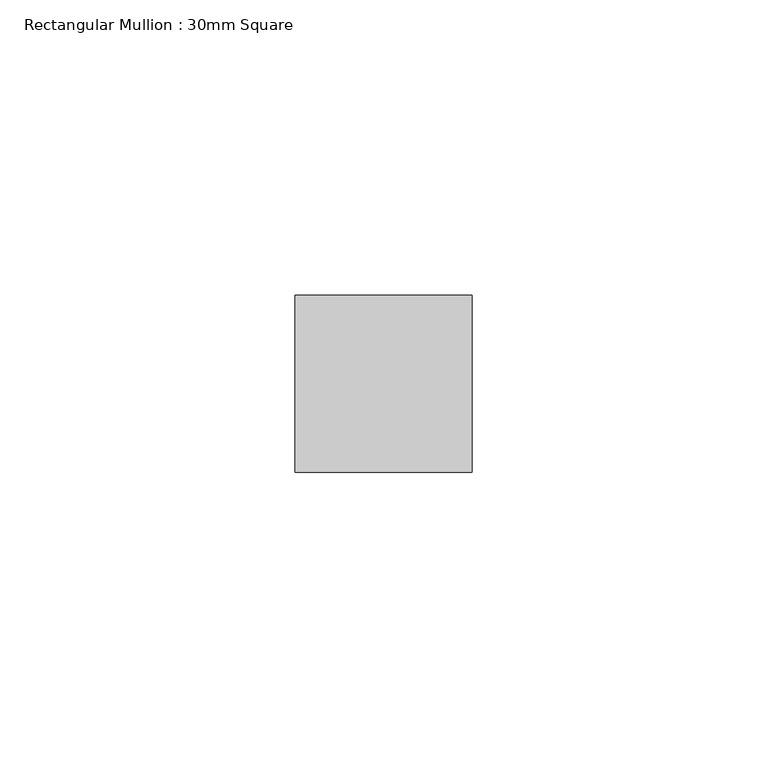
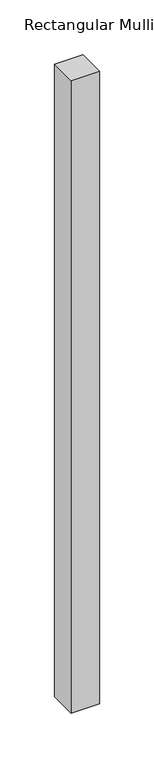
"""IFC4 building model written with IfcOpenShell, lengths in millimetres: member geometry, Rectangular Mullion : 30mm Square."""

from ifc_helpers import new_model, si_unit, frame, origin, place, context, project, spatial, polyline, outline, extrude, source, transform, mapped, element, save


def rectangular_mullion_30mm_square_4c7eb74d(model_context):
    return source(origin(), model_context, "Body", "SweptSolid", [
        extrude(outline(polyline([(15.0, 15.0), (15.0, -15.0), (-15.0, -15.0), (-15.0, 15.0), (15.0, 15.0)])), frame((0.0, 0.0, -705.0), z_axis=(0.0, 0.0, 1.0), x_axis=(1.0, 0.0, 0.0)), (0.0, 0.0, 1.0), 705.0),
    ])


if __name__ == "__main__":
    model = new_model("IFC4")
    model_context = context("Model", 3, world=origin())
    ifc_project = project(units=[si_unit("LENGTHUNIT", "METRE", prefix="MILLI")], contexts=[model_context])
    site = spatial("IfcSite", under=ifc_project)
    building = spatial("IfcBuilding", under=site)
    placement = place(None, origin())
    rectangular_mullion_30mm_square_shape = rectangular_mullion_30mm_square_4c7eb74d(model_context)
    element("IfcMember", 1, ObjectType="Rectangular Mullion : 30mm Square", at=placement, inside=building, context=model_context, shape_type="MappedRepresentation", body=[
        mapped(rectangular_mullion_30mm_square_shape, transform((0.0, 0.0, 0.0), x_axis=(1.0, 0.0, 0.0), y_axis=(0.0, 1.0, 0.0), z_axis=(0.0, 0.0, 1.0))),
    ])
    save(model, "model.ifc")

# Revit data of these elements
# Type "Rectangular Mullion : 30mm Square"
#   built-in parameter 1007304 = 0.0984252 (stored number, unit not read)
#   built-in parameter 1007301 = 0.0492126 (stored number, unit not read)
#   built-in parameter 1007300 = 0.0492126 (stored number, unit not read)
# Element 1 (IfcMember, "Rectangular Mullion : 30mm Square")
#   Materials on its faces: "Aluminum"
# Materials
#   "Aluminum": class "Metal", colour RGB 244 244 244, transparency 0, Description = "Aluminum 6061", Cost = 0
